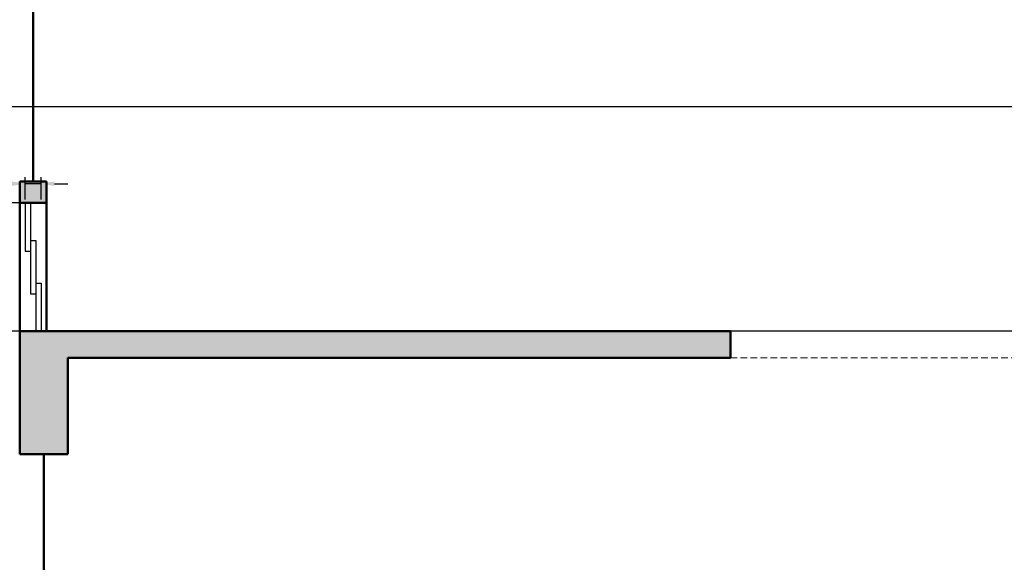
# Model space of a CAD drawing. Units: inches. Extents: x 1913 to 5309, y 1003 to 1733.
# Tile 15 of 23: x 4152 to 4336, y 1286 to 1387. Entities that reach past the tile are written whole.
import ezdxf

# ---------------------------------------------------------------- set-up
doc = ezdxf.new("R2010")
doc.units = ezdxf.units.IN
doc.linetypes.add('HIDDEN2', pattern=[0.1875, 0.125, -0.0625])
for name, color, linetype, lineweight in [('A-ANNO-DIMS', 2, 'Continuous', 18), ('A-FLOR-PATT', 252, 'Continuous', 13), ('A-GLAZ', 5, 'Continuous', 25), ('A-WALL', 7, 'Continuous', 50), ('A-WALL-OVHD', 8, 'HIDDEN2', 18)]:
    doc.layers.add(name, color=color, linetype=linetype, lineweight=lineweight)
doc.styles.get("Standard").update_dxf_attribs({"font": 'arial.ttf'})
doc.dimstyles.new('ISO-25', dxfattribs={"dimtxt": 8, "dimasz": 2.5, "dimexe": 1.25, "dimexo": 0.625, "dimtad": 1, "dimdec": 1, "dimlunit": 3, "dimtxsty": 'Standard', "dimcen": 2.5, "dimclrd": 256, "dimclrt": 1, "dimadec": 0, "dimazin": 0, "dimtfac": 1, "dimtdec": 1, "dimtmove": 0, "dimatfit": 3, "dimfxl": 1, "dimarcsym": 0})

# ---------------------------------------------------------------- blocks, each defined once
blk = doc.blocks.new('WIN-24')
for p, q in [((0, 15), (0, 24)), ((1, 7), (1, 24)), ((2, 17), (1, 17)), ((2, 0), (2, 17)), ((1, 15), (0, 15)), ((3, 9), (2, 9)), ((3, 0), (3, 9)), ((2, 7), (1, 7))]:
    blk.add_line(p, q)
blk = doc.blocks.new('*D59')
at = {"layer": 'A-ANNO-DIMS', "color": 0, "lineweight": -2, "transparency": 16777216}
for p, q in [((4152.59, 1352.96), (4148.36, 1352.96)), ((4152.59, 1328.96), (4148.36, 1328.96))]:
    blk.add_line(p, q, dxfattribs=at)
at = {"layer": 'A-ANNO-DIMS', "lineweight": -2, "transparency": 16777216}
for p, q in [((4149.61, 1350.46), (4149.61, 1331.46)), ((4149.61, 1328.96), (4149.61, 1223.98))]:
    blk.add_line(p, q, dxfattribs=at)
at = {"layer": 'A-ANNO-DIMS', "transparency": 16777216}
for points in [[(4149.2, 1350.46), (4150.03, 1350.46), (4149.61, 1352.96)], [(4149.2, 1331.46), (4150.03, 1331.46), (4149.61, 1328.96)]]:
    blk.add_solid(points, dxfattribs=at)
at = {"layer": 'Defpoints', "color": 0, "transparency": 16777216}
for p in [(4153.21, 1352.96), (4149.61, 1328.96), (4153.21, 1328.96)]:
    blk.add_point(p, dxfattribs=at)
at = {"layer": 'A-ANNO-DIMS', "color": 1, "transparency": 16777216, "insert": (4144.85, 1275.22), "char_height": 8, "attachment_point": 5, "rotation": 90}
blk.add_mtext('WINDOW 2\'-0" TYP.', dxfattribs=at)
blk = doc.blocks.new('*D60')
at = {"layer": 'A-ANNO-DIMS', "color": 0, "lineweight": -2, "transparency": 16777216}
for p, q in [((4153.21, 1353.59), (4153.21, 1357.81)), ((4156.21, 1353.59), (4156.21, 1357.81))]:
    blk.add_line(p, q, dxfattribs=at)
at = {"layer": 'A-ANNO-DIMS', "lineweight": -2, "transparency": 16777216}
for p, q in [((4150.71, 1356.56), (4098.2, 1356.56)), ((4156.21, 1356.56), (4153.21, 1356.56)), ((4158.71, 1356.56), (4161.21, 1356.56))]:
    blk.add_line(p, q, dxfattribs=at)
at = {"layer": 'A-ANNO-DIMS', "transparency": 16777216}
for points in [[(4150.71, 1356.98), (4150.71, 1356.15), (4153.21, 1356.56)], [(4158.71, 1356.98), (4158.71, 1356.15), (4156.21, 1356.56)]]:
    blk.add_solid(points, dxfattribs=at)
at = {"layer": 'Defpoints', "color": 0, "transparency": 16777216}
for p in [(4153.21, 1356.56), (4153.21, 1352.96), (4156.21, 1352.96)]:
    blk.add_point(p, dxfattribs=at)
at = {"layer": 'A-ANNO-DIMS', "color": 1, "transparency": 16777216, "insert": (4123.21, 1361.28), "char_height": 8, "attachment_point": 5}
blk.add_mtext('0\'-3" TYP.', dxfattribs=at)
blk = doc.blocks.new('*D115')
at = {"layer": 'A-ANNO-DIMS', "color": 0, "lineweight": -2, "transparency": 16777216}
for p, q in [((4416.59, 1370.96), (3925.96, 1370.96)), ((4416.59, 1328.96), (3925.96, 1328.96))]:
    blk.add_line(p, q, dxfattribs=at)
at = {"layer": 'A-ANNO-DIMS', "lineweight": -2, "transparency": 16777216}
blk.add_line((3927.21, 1331.46), (3927.21, 1368.46), dxfattribs=at)
at = {"layer": 'A-ANNO-DIMS', "transparency": 16777216}
for points in [[(3926.8, 1368.46), (3927.63, 1368.46), (3927.21, 1370.96)], [(3926.8, 1331.46), (3927.63, 1331.46), (3927.21, 1328.96)]]:
    blk.add_solid(points, dxfattribs=at)
at = {"layer": 'Defpoints', "color": 0, "transparency": 16777216}
for p in [(3927.21, 1370.96), (4417.21, 1370.96), (4417.21, 1328.96)]:
    blk.add_point(p, dxfattribs=at)
at = {"layer": 'A-ANNO-DIMS', "color": 1, "transparency": 16777216, "insert": (3922.5, 1349.96), "char_height": 8, "attachment_point": 5, "rotation": 90}
blk.add_mtext('3\'-6"', dxfattribs=at)

msp = doc.modelspace()

# ---------------------------------------------------------------- hatches: boundary and pattern name
at = {"layer": 'A-FLOR-PATT'}
h = msp.add_hatch(color=256, dxfattribs=at)
h.dxf.hatch_style = 1
h.paths.add_polyline_path([(4179.21, 1155.93), (4164.35, 1155.93, -0.035946), (4163.9, 1155.96), (4161.21, 1155.96), (4161.21, 1173.96), (4152.21, 1173.96), (4152.21, 1146.96), (4179.21, 1146.96)])
h.paths.add_polyline_path([(4273.21, 1155.96), (4266.93, 1155.96), (4233.21, 1155.96), (4233.21, 1146.96), (4273.21, 1146.96)])
h.paths.add_polyline_path([(4285.21, 1328.96), (4152.21, 1328.96), (4152.21, 1305.96), (4161.21, 1305.96), (4161.21, 1323.96), (4285.21, 1323.96)])
h.paths.add_polyline_path([(4161.21, 1257.96), (4152.21, 1257.96), (4152.21, 1233.96), (4161.21, 1233.96), (4161.21, 1237.71)])
h.paths.add_polyline_path([(4515.21, 1405.96), (4503.21, 1405.96), (4503.21, 1400.96), (4506.21, 1400.96), (4506.21, 1328.96), (4452.21, 1328.96), (4452.21, 1323.96), (4506.21, 1323.96), (4506.21, 1179.96), (4455.21, 1179.96), (4455.21, 1170.96), (4515.21, 1170.96)])
h.paths.add_polyline_path([(4157.21, 1686.96), (3999.21, 1686.96), (3999.21, 1625.96), (4008.21, 1625.96), (4008.21, 1677.96), (4152.21, 1677.96), (4152.21, 1554.96), (4157.21, 1554.96), (4157.21, 1599.96), (4225.21, 1599.96), (4225.21, 1608.96), (4157.21, 1608.96)])
h.paths.add_polyline_path([(4008.21, 1513.96), (4157.21, 1513.96), (4157.21, 1518.96), (4008.21, 1518.96), (4008.21, 1571.96), (3999.21, 1571.96), (3999.21, 1420.96), (4050.21, 1420.96), (4050.21, 1429.96), (4008.21, 1429.96)])
h.paths.add_polyline_path([(4157.21, 1477.96), (4152.21, 1477.96), (4152.21, 1429.96), (4110.21, 1429.96), (4110.21, 1420.96), (4157.21, 1420.96)], flags=17)
h.paths.add_polyline_path([(4350.21, 1608.96), (4345.21, 1608.96), (4321.21, 1608.96), (4321.21, 1599.96), (4350.21, 1599.96)])
h.paths.add_polyline_path([(4515.21, 1686.96), (4345.21, 1686.96), (4345.21, 1644.96), (4350.21, 1644.96), (4350.21, 1677.96), (4506.21, 1677.96), (4506.21, 1557.96), (4423.21, 1557.96), (4423.21, 1552.96), (4506.21, 1552.96), (4506.21, 1492.96), (4428.21, 1492.96), (4428.21, 1522.96), (4423.21, 1522.96), (4423.21, 1492.96), (4345.21, 1492.96), (4345.21, 1487.96), (4474.21, 1487.96), (4474.21, 1464.96), (4479.21, 1464.96), (4479.21, 1487.96), (4515.21, 1487.96)])
h.paths.add_polyline_path([(4479.21, 1428.96), (4474.21, 1428.96), (4474.21, 1405.96), (4345.21, 1405.96), (4345.21, 1358.96), (4350.21, 1358.96), (4350.21, 1400.96), (4417.21, 1400.96), (4417.21, 1394.96), (4422.21, 1394.96), (4422.21, 1400.96), (4479.21, 1400.96)])
h.paths.add_polyline_path([(4350.21, 1323.96), (4422.21, 1323.96), (4422.21, 1370.96), (4417.21, 1370.96), (4417.21, 1328.96), (4345.21, 1328.96), (4345.21, 1158.97, -0.414214), (4342.21, 1155.96), (4327.21, 1155.96), (4327.21, 1146.96), (4350.21, 1146.96), (4350.21, 1170.96), (4401.21, 1170.96), (4401.21, 1179.96), (4350.21, 1179.96)])
h.paths.add_polyline_path([(4157.21, 1356.96), (4152.21, 1356.96), (4152.21, 1352.96), (4157.21, 1352.96)])
h.paths.add_polyline_path([(4157.21, 1396.96), (4152.21, 1396.96), (4152.21, 1392.96), (4157.21, 1392.96)])

# ---------------------------------------------------------------- linework, layer by layer
at = {"layer": 'A-WALL'}
for p, q in [((4154.71, 1392.96), (4154.71, 1356.96)), ((4152.21, 1356.96), (4157.21, 1356.96)), ((4152.21, 1356.96), (4152.21, 1305.96)), ((4157.21, 1356.96), (4157.21, 1328.96)), ((4152.21, 1352.96), (4157.21, 1352.96)), ((4152.21, 1328.96), (4285.21, 1328.96)), ((4285.21, 1328.96), (4285.21, 1323.96)), ((4161.21, 1323.96), (4285.21, 1323.96)), ((4161.21, 1323.96), (4161.21, 1305.96)), ((4152.21, 1305.96), (4161.21, 1305.96)), ((4156.71, 1305.96), (4156.71, 1257.96))]:
    msp.add_line(p, q, dxfattribs=at)
at = {"layer": 'A-WALL-OVHD', "ltscale": 10}
for p, q in [((4285.21, 1328.96), (4345.21, 1328.96)), ((4285.21, 1323.96), (4345.21, 1323.96))]:
    msp.add_line(p, q, dxfattribs=at)

# ---------------------------------------------------------------- block references
at = {"layer": 'A-GLAZ', "rotation": 180}
msp.add_blockref('WIN-24', (4156.21, 1352.96), dxfattribs=at)

# ---------------------------------------------------------------- dimensions: what is measured, and where the dimension line sits
at = {"layer": 'A-ANNO-DIMS'}
for base, p1, p2, angle, text, picture, middle in [((4153.21, 1356.56), (4156.21, 1352.96), (4153.21, 1352.96), 180, '<> TYP.', '*D60', (4123.21, 1361.28)), ((4149.61, 1328.96), (4153.21, 1352.96), (4153.21, 1328.96), 270, 'WINDOW <> TYP.', '*D59', (4144.85, 1275.22))]:
    dim = msp.add_linear_dim(base=base, p1=p1, p2=p2, angle=angle, text=text, dimstyle='ISO-25', override={"dimdec": 1, "dimrnd": 0, "dimzin": 1, "dimlunit": 4, "dimfrac": 2}, dxfattribs=at)
    dim.commit()
    dim.dimension.update_dxf_attribs({"geometry": picture, "text_midpoint": middle})
dim = msp.add_linear_dim(base=(3927.21, 1370.96), p1=(4417.21, 1328.96), p2=(4417.21, 1370.96), angle=90, dimstyle='ISO-25', override={"dimdec": 1, "dimlfac": 1, "dimrnd": 0, "dimzin": 1, "dimdsep": 46, "dimlunit": 4, "dimfrac": 2}, dxfattribs=at)
dim.commit()
dim.dimension.update_dxf_attribs({"geometry": '*D115', "text_midpoint": (3922.5, 1349.96)})

doc.saveas('drawing.dxf')
